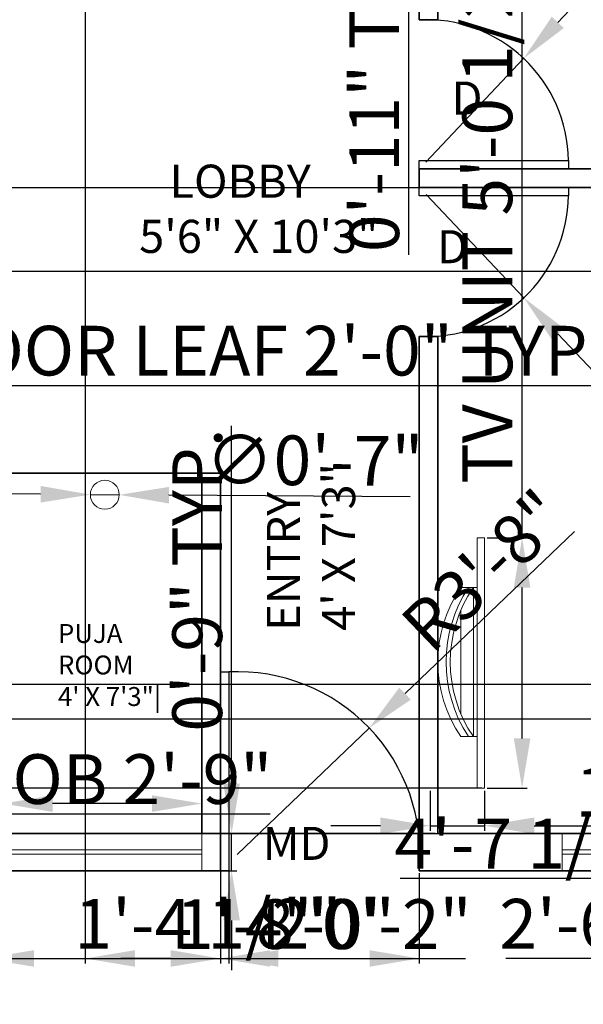
# Model space of a CAD drawing. Units: inches. Extents: x 2122 to 2726, y 1923 to 2370.
# Tile 2 of 6: x 2370 to 2506, y 1940 to 2178. Entities that reach past the tile are written whole.
import ezdxf

# ---------------------------------------------------------------- set-up
doc = ezdxf.new("R2010")
doc.units = ezdxf.units.IN
for name, color, linetype, lineweight in [('A-ANNO-DIMS', 2, 'Continuous', 18), ('A-ANNO-TEXT', 7, 'Continuous', 18), ('A-AREA-IDEN', 7, 'Continuous', 25), ('A-DOOR', 3, 'Continuous', 25), ('A-EQPM', 9, 'Continuous', 18), ('A-FLOR-FIXT', 9, 'Continuous', 18), ('A-GLAZ', 4, 'Continuous', 18), ('A-WALL', 7, 'Continuous', 35)]:
    doc.layers.add(name, color=color, linetype=linetype, lineweight=lineweight)
doc.styles.get("Standard").update_dxf_attribs({"font": 'arial.ttf'})
doc.dimstyles.new('ISO-25', dxfattribs={"dimtxt": 12, "dimasz": 12, "dimexe": 1.25, "dimexo": 0.625, "dimtad": 1, "dimlunit": 3, "dimtxsty": 'Standard', "dimcen": 2.5, "dimadec": 0, "dimazin": 0, "dimtfac": 1, "dimtmove": 0, "dimatfit": 3, "dimfxl": 1, "dimarcsym": 0})

# ---------------------------------------------------------------- blocks, each defined once
blk = doc.blocks.new('Television')
for p, q in [((2488.56, 2041.12), (2484.64, 2041.12)), ((2487.64, 2005.12), (2487.64, 2041.12)), ((2484.64, 2010.57), (2484.64, 2035.66)), ((2488.56, 2005.12), (2484.64, 2005.12))]:
    blk.add_line(p, q)
blk.add_lwpolyline([(2488.56, 2053.12), (2490.33, 2053.12), (2490.33, 1992.66), (2488.56, 1992.66)], close=True)
for centre, radius, start, end in [((2510.99, 2023.12), 31.91, 145.6614, 214.3386), ((2513.92, 2023.12), 32.85, 146.7698, 213.2302), ((2513.92, 2023.12), 31.85, 145.583, 214.417)]:
    blk.add_arc(centre, radius, start, end)
blk = doc.blocks.new('WIN-60IN')
for p, q in [((0, 0), (0, 9)), ((60, 0), (60, 9)), ((0, 5), (60, 5)), ((0, 4), (60, 4))]:
    blk.add_line(p, q)
blk = doc.blocks.new('WIN-48IN')
for p, q in [((9, 48), (0, 48)), ((4, 0), (4, 48)), ((5, 0), (5, 48)), ((9, 0), (0, 0))]:
    blk.add_line(p, q)
blk = doc.blocks.new('DOOR-LEAF-36IN')
for p, q in [((0, 2), (36, 2)), ((0, 0), (0, 2)), ((36, 0), (0, 0)), ((36, 2), (36, 0))]:
    blk.add_line(p, q)
blk = doc.blocks.new('*D18')
at = {"layer": 'A-ANNO-DIMS', "color": 0, "lineweight": -2, "transparency": 16777216}
for p, q in [((2366.01, 1982.36), (2366.01, 1990.19)), ((2414.01, 1982.36), (2414.01, 1990.19)), ((2366.01, 1988.94), (2200.91, 1988.94)), ((2402.01, 1988.94), (2378.01, 1988.94))]:
    blk.add_line(p, q, dxfattribs=at)
at = {"layer": 'A-ANNO-DIMS', "color": 0, "transparency": 16777216}
for points in [[(2378.01, 1990.94), (2378.01, 1986.94), (2366.01, 1988.94)], [(2402.01, 1990.94), (2402.01, 1986.94), (2414.01, 1988.94)]]:
    blk.add_solid(points, dxfattribs=at)
at = {"layer": 'Defpoints', "color": 0, "transparency": 16777216}
for p in [(2366.01, 1988.94), (2366.01, 1981.74), (2414.01, 1981.74)]:
    blk.add_point(p, dxfattribs=at)
at = {"layer": 'A-ANNO-DIMS', "color": 0, "transparency": 16777216, "insert": (2277.46, 1995.77), "char_height": 12, "attachment_point": 5}
blk.add_mtext('WINDOW 4\'-0" TYP.', dxfattribs=at)
blk = doc.blocks.new('*D19')
at = {"layer": 'A-ANNO-DIMS', "color": 0, "lineweight": -2, "transparency": 16777216}
for p, q in [((2421.21, 1993.74), (2421.21, 2080.13)), ((2414.63, 1981.74), (2422.46, 1981.74)), ((2421.21, 1972.74), (2421.21, 1981.74)), ((2414.63, 1972.74), (2422.46, 1972.74)), ((2421.21, 1960.74), (2421.21, 1948.74))]:
    blk.add_line(p, q, dxfattribs=at)
at = {"layer": 'A-ANNO-DIMS', "color": 0, "transparency": 16777216}
for points in [[(2419.21, 1993.74), (2423.21, 1993.74), (2421.21, 1981.74)], [(2419.21, 1960.74), (2423.21, 1960.74), (2421.21, 1972.74)]]:
    blk.add_solid(points, dxfattribs=at)
at = {"layer": 'Defpoints', "color": 0, "transparency": 16777216}
for p in [(2414.01, 1981.74), (2421.21, 1981.74), (2414.01, 1972.74)]:
    blk.add_point(p, dxfattribs=at)
at = {"layer": 'A-ANNO-DIMS', "color": 0, "transparency": 16777216, "insert": (2414.46, 2042.93), "char_height": 12, "attachment_point": 5, "rotation": 90}
blk.add_mtext('0\'-9" TYP.', dxfattribs=at)
blk = doc.blocks.new('*D24')
at = {"layer": 'A-ANNO-DIMS', "color": 0, "lineweight": -2, "transparency": 16777216}
for p, q in [((2294.01, 2092.91), (2294.01, 2088.68)), ((2318.01, 2092.91), (2318.01, 2088.68)), ((2282.01, 2089.93), (2270.01, 2089.93)), ((2294.01, 2089.93), (2318.01, 2089.93)), ((2330.01, 2089.93), (2517.34, 2089.93))]:
    blk.add_line(p, q, dxfattribs=at)
at = {"layer": 'A-ANNO-DIMS', "color": 0, "transparency": 16777216}
for points in [[(2282.01, 2091.93), (2282.01, 2087.93), (2294.01, 2089.93)], [(2330.01, 2091.93), (2330.01, 2087.93), (2318.01, 2089.93)]]:
    blk.add_solid(points, dxfattribs=at)
at = {"layer": 'Defpoints', "color": 0, "transparency": 16777216}
for p in [(2294.01, 2093.53), (2318.01, 2093.53), (2318.01, 2089.93)]:
    blk.add_point(p, dxfattribs=at)
at = {"layer": 'A-ANNO-DIMS', "color": 0, "transparency": 16777216, "insert": (2429.67, 2096.76), "char_height": 12, "attachment_point": 5}
blk.add_mtext('DOOR LEAF 2\'-0" TYP.', dxfattribs=at)
blk = doc.blocks.new('*D29')
at = {"layer": 'A-ANNO-DIMS', "color": 0, "lineweight": -2, "transparency": 16777216}
for p, q in [((2463.94, 2251.92), (2463.94, 2263.92)), ((2462.8, 2239.92), (2465.19, 2239.92)), ((2463.94, 2239.92), (2463.94, 2229.14)), ((2462.8, 2229.14), (2465.19, 2229.14)), ((2463.94, 2217.14), (2463.94, 2121.42))]:
    blk.add_line(p, q, dxfattribs=at)
at = {"layer": 'A-ANNO-DIMS', "color": 0, "transparency": 16777216}
for points in [[(2461.94, 2251.92), (2465.94, 2251.92), (2463.94, 2239.92)], [(2461.94, 2217.14), (2465.94, 2217.14), (2463.94, 2229.14)]]:
    blk.add_solid(points, dxfattribs=at)
at = {"layer": 'Defpoints', "color": 0, "transparency": 16777216}
for p in [(2462.17, 2239.92), (2462.17, 2229.14), (2463.94, 2229.14)]:
    blk.add_point(p, dxfattribs=at)
at = {"layer": 'A-ANNO-DIMS', "color": 0, "transparency": 16777216, "insert": (2457.19, 2163.28), "char_height": 12, "attachment_point": 5, "rotation": 90}
blk.add_mtext('0\'-11" TYP.', dxfattribs=at)
blk = doc.blocks.new('*D30')
at = {"layer": 'A-ANNO-DIMS', "color": 0, "lineweight": -2, "transparency": 16777216}
for p, q in [((2311.94, 1990.8), (2311.94, 1985.22)), ((2344.99, 1990.8), (2344.99, 1985.22)), ((2323.94, 1986.47), (2332.99, 1986.47)), ((2344.99, 1986.47), (2430.48, 1986.47))]:
    blk.add_line(p, q, dxfattribs=at)
at = {"layer": 'A-ANNO-DIMS', "color": 0, "transparency": 16777216}
for points in [[(2323.94, 1988.47), (2323.94, 1984.47), (2311.94, 1986.47)], [(2332.99, 1988.47), (2332.99, 1984.47), (2344.99, 1986.47)]]:
    blk.add_solid(points, dxfattribs=at)
at = {"layer": 'Defpoints', "color": 0, "transparency": 16777216}
for p in [(2311.94, 1991.43), (2344.99, 1991.43), (2344.99, 1986.47)]:
    blk.add_point(p, dxfattribs=at)
at = {"layer": 'A-ANNO-DIMS', "color": 0, "transparency": 16777216, "insert": (2393.73, 1993.3), "char_height": 12, "attachment_point": 5}
blk.add_mtext('HOB 2\'-9"', dxfattribs=at)
blk = doc.blocks.new('*D34')
at = {"layer": 'A-ANNO-DIMS', "color": 0, "lineweight": -2, "transparency": 16777216}
for p, q in [((2524.67, 2054.11), (2524.67, 2177.46)), ((2534.9, 2054.11), (2523.42, 2054.11)), ((2524.67, 1993.74), (2524.67, 2042.11)), ((2534.9, 1981.74), (2523.42, 1981.74))]:
    blk.add_line(p, q, dxfattribs=at)
at = {"layer": 'A-ANNO-DIMS', "color": 0, "transparency": 16777216}
for points in [[(2522.67, 2042.11), (2526.67, 2042.11), (2524.67, 2054.11)], [(2522.67, 1993.74), (2526.67, 1993.74), (2524.67, 1981.74)]]:
    blk.add_solid(points, dxfattribs=at)
at = {"layer": 'Defpoints', "color": 0, "transparency": 16777216}
for p in [(2524.67, 2054.11), (2535.52, 2054.11), (2535.52, 1981.74)]:
    blk.add_point(p, dxfattribs=at)
at = {"layer": 'A-ANNO-DIMS', "color": 0, "transparency": 16777216, "insert": (2517.83, 2121.79), "char_height": 12, "attachment_point": 5, "rotation": 90}
blk.add_mtext('SOFA 6\'-0 1/2"', dxfattribs=at)
blk = doc.blocks.new('*D35')
at = {"layer": 'A-ANNO-DIMS', "color": 0, "lineweight": -2, "transparency": 16777216}
for p, q in [((2535.52, 1981.11), (2535.52, 1969.63)), ((2591.01, 1981.11), (2591.01, 1969.63)), ((2535.52, 1970.88), (2461.93, 1970.88)), ((2579.01, 1970.88), (2547.52, 1970.88))]:
    blk.add_line(p, q, dxfattribs=at)
at = {"layer": 'A-ANNO-DIMS', "color": 0, "transparency": 16777216}
for points in [[(2547.52, 1972.88), (2547.52, 1968.88), (2535.52, 1970.88)], [(2579.01, 1972.88), (2579.01, 1968.88), (2591.01, 1970.88)]]:
    blk.add_solid(points, dxfattribs=at)
at = {"layer": 'Defpoints', "color": 0, "transparency": 16777216}
for p in [(2535.52, 1981.74), (2591.01, 1981.74), (2535.52, 1970.88)]:
    blk.add_point(p, dxfattribs=at)
at = {"layer": 'A-ANNO-DIMS', "color": 0, "transparency": 16777216, "insert": (2492.72, 1977.71), "char_height": 12, "attachment_point": 5}
blk.add_mtext('4\'-7 1/2"', dxfattribs=at)
blk = doc.blocks.new('*D36')
at = {"layer": 'A-ANNO-DIMS', "color": 0, "lineweight": -2, "transparency": 16777216}
for p, q in [((2491.33, 2053.12), (2491.33, 2196.38)), ((2482.88, 2053.12), (2492.58, 2053.12)), ((2491.33, 2004.66), (2491.33, 2041.12)), ((2482.88, 1992.66), (2492.58, 1992.66))]:
    blk.add_line(p, q, dxfattribs=at)
at = {"layer": 'A-ANNO-DIMS', "color": 0, "transparency": 16777216}
for points in [[(2489.33, 2041.12), (2493.33, 2041.12), (2491.33, 2053.12)], [(2489.33, 2004.66), (2493.33, 2004.66), (2491.33, 1992.66)]]:
    blk.add_solid(points, dxfattribs=at)
at = {"layer": 'Defpoints', "color": 0, "transparency": 16777216}
for p in [(2482.26, 2053.12), (2491.33, 2053.12), (2482.26, 1992.66)]:
    blk.add_point(p, dxfattribs=at)
at = {"layer": 'A-ANNO-DIMS', "color": 0, "transparency": 16777216, "insert": (2484.5, 2130.75), "char_height": 12, "attachment_point": 5, "rotation": 90}
blk.add_mtext('TV UNIT 5\'-0 1/2"', dxfattribs=at)
blk = doc.blocks.new('*D37')
at = {"layer": 'A-ANNO-DIMS', "color": 0, "lineweight": -2, "transparency": 16777216}
for p, q in [((2469.15, 1992.03), (2469.15, 1982.34)), ((2482.26, 1992.03), (2482.26, 1982.34)), ((2457.15, 1983.59), (2445.15, 1983.59)), ((2469.15, 1983.59), (2482.26, 1983.59)), ((2494.26, 1983.59), (2538.28, 1983.59))]:
    blk.add_line(p, q, dxfattribs=at)
at = {"layer": 'A-ANNO-DIMS', "color": 0, "transparency": 16777216}
for points in [[(2457.15, 1985.59), (2457.15, 1981.59), (2469.15, 1983.59)], [(2494.26, 1985.59), (2494.26, 1981.59), (2482.26, 1983.59)]]:
    blk.add_solid(points, dxfattribs=at)
at = {"layer": 'Defpoints', "color": 0, "transparency": 16777216}
for p in [(2469.15, 1992.66), (2482.26, 1992.66), (2482.26, 1983.59)]:
    blk.add_point(p, dxfattribs=at)
at = {"layer": 'A-ANNO-DIMS', "color": 0, "transparency": 16777216, "insert": (2522.27, 1990.24), "char_height": 12, "attachment_point": 5}
blk.add_mtext('1\'-1"', dxfattribs=at)
blk = doc.blocks.new('*D38')
at = {"layer": 'A-ANNO-DIMS', "color": 0, "lineweight": -2, "transparency": 16777216}
for p, q in [((2418.51, 1972.11), (2418.51, 1950.29)), ((2466.51, 1972.11), (2466.51, 1950.29)), ((2430.51, 1951.54), (2454.51, 1951.54))]:
    blk.add_line(p, q, dxfattribs=at)
at = {"layer": 'A-ANNO-DIMS', "color": 0, "transparency": 16777216}
for points in [[(2430.51, 1953.54), (2430.51, 1949.54), (2418.51, 1951.54)], [(2454.51, 1953.54), (2454.51, 1949.54), (2466.51, 1951.54)]]:
    blk.add_solid(points, dxfattribs=at)
at = {"layer": 'Defpoints', "color": 0, "transparency": 16777216}
for p in [(2418.51, 1972.74), (2466.51, 1972.74), (2466.51, 1951.54)]:
    blk.add_point(p, dxfattribs=at)
at = {"layer": 'A-ANNO-DIMS', "color": 0, "transparency": 16777216, "insert": (2442.51, 1958.29), "char_height": 12, "attachment_point": 5}
blk.add_mtext('4\'-0"', dxfattribs=at)
blk = doc.blocks.new('*D40')
at = {"layer": 'A-ANNO-DIMS', "color": 0, "lineweight": -2, "transparency": 16777216}
for p, q in [((2362.13, 2017.74), (2622.46, 2017.74)), ((2621.21, 1993.74), (2621.21, 2005.74)), ((2362.13, 1981.74), (2622.46, 1981.74))]:
    blk.add_line(p, q, dxfattribs=at)
at = {"layer": 'A-ANNO-DIMS', "color": 0, "transparency": 16777216}
for points in [[(2619.21, 2005.74), (2623.21, 2005.74), (2621.21, 2017.74)], [(2619.21, 1993.74), (2623.21, 1993.74), (2621.21, 1981.74)]]:
    blk.add_solid(points, dxfattribs=at)
at = {"layer": 'Defpoints', "color": 0, "transparency": 16777216}
for p in [(2361.51, 2017.74), (2621.21, 2017.74), (2361.51, 1981.74)]:
    blk.add_point(p, dxfattribs=at)
at = {"layer": 'A-ANNO-DIMS', "color": 0, "transparency": 16777216, "insert": (2614.45, 1999.74), "char_height": 12, "attachment_point": 5, "rotation": 90}
blk.add_mtext('3\'-0"', dxfattribs=at)
blk = doc.blocks.new('*D50')
at = {"layer": 'A-ANNO-DIMS', "color": 0, "lineweight": -2, "transparency": 16777216}
for p, q in [((2366.01, 2189.61), (2366.01, 1950.29)), ((2385.88, 2189.61), (2385.88, 1950.29)), ((2354.01, 1951.54), (2342.01, 1951.54)), ((2366.01, 1951.54), (2385.88, 1951.54)), ((2397.88, 1951.54), (2441.9, 1951.54))]:
    blk.add_line(p, q, dxfattribs=at)
at = {"layer": 'A-ANNO-DIMS', "color": 0, "transparency": 16777216}
for points in [[(2354.01, 1953.54), (2354.01, 1949.54), (2366.01, 1951.54)], [(2397.88, 1953.54), (2397.88, 1949.54), (2385.88, 1951.54)]]:
    blk.add_solid(points, dxfattribs=at)
at = {"layer": 'Defpoints', "color": 0, "transparency": 16777216}
for p in [(2366.01, 2190.24), (2385.88, 2190.24), (2385.88, 1951.54)]:
    blk.add_point(p, dxfattribs=at)
at = {"layer": 'A-ANNO-DIMS', "color": 0, "transparency": 16777216, "insert": (2425.89, 1958.29), "char_height": 12, "attachment_point": 5}
blk.add_mtext('1\'-8"', dxfattribs=at)
blk = doc.blocks.new('*D51')
at = {"layer": 'A-ANNO-DIMS', "color": 0, "lineweight": -2, "transparency": 16777216}
for p, q in [((2211.31, 2209.57), (2211.31, 2282.68)), ((2465.88, 2197.57), (2210.06, 2197.57)), ((2211.31, 2190.24), (2211.31, 2197.57)), ((2465.88, 2190.24), (2210.06, 2190.24)), ((2211.31, 2178.24), (2211.31, 2166.24))]:
    blk.add_line(p, q, dxfattribs=at)
at = {"layer": 'A-ANNO-DIMS', "color": 0, "transparency": 16777216}
for points in [[(2209.31, 2209.57), (2213.31, 2209.57), (2211.31, 2197.57)], [(2209.31, 2178.24), (2213.31, 2178.24), (2211.31, 2190.24)]]:
    blk.add_solid(points, dxfattribs=at)
at = {"layer": 'Defpoints', "color": 0, "transparency": 16777216}
for p in [(2211.31, 2197.57), (2466.51, 2197.57), (2466.51, 2190.24)]:
    blk.add_point(p, dxfattribs=at)
at = {"layer": 'A-ANNO-DIMS', "color": 0, "transparency": 16777216, "insert": (2204.48, 2252.12), "char_height": 12, "attachment_point": 5, "rotation": 90}
blk.add_mtext('0\'-7 1/2"', dxfattribs=at)
blk = doc.blocks.new('*D52')
at = {"layer": 'A-ANNO-DIMS', "color": 0, "lineweight": -2, "transparency": 16777216}
for p, q in [((2621.21, 2149.74), (2621.21, 2161.74)), ((2314.13, 2137.74), (2622.46, 2137.74)), ((2621.21, 2137.74), (2621.21, 2117.53)), ((2314.13, 2117.53), (2622.46, 2117.53)), ((2621.21, 2105.53), (2621.21, 2061.51))]:
    blk.add_line(p, q, dxfattribs=at)
at = {"layer": 'A-ANNO-DIMS', "color": 0, "transparency": 16777216}
for points in [[(2619.21, 2149.74), (2623.21, 2149.74), (2621.21, 2137.74)], [(2619.21, 2105.53), (2623.21, 2105.53), (2621.21, 2117.53)]]:
    blk.add_solid(points, dxfattribs=at)
at = {"layer": 'Defpoints', "color": 0, "transparency": 16777216}
for p in [(2313.51, 2137.74), (2313.51, 2117.53), (2621.21, 2117.53)]:
    blk.add_point(p, dxfattribs=at)
at = {"layer": 'A-ANNO-DIMS', "color": 0, "transparency": 16777216, "insert": (2614.46, 2077.52), "char_height": 12, "attachment_point": 5, "rotation": 90}
blk.add_mtext('1\'-8"', dxfattribs=at)
blk = doc.blocks.new('*D55')
at = {"layer": 'A-ANNO-DIMS', "color": 0, "lineweight": -2, "transparency": 16777216}
for p, q in [((2344.97, 1990.8), (2344.97, 1950.29)), ((2361.51, 1981.11), (2361.51, 1950.29)), ((2332.97, 1951.54), (2320.97, 1951.54)), ((2344.97, 1951.54), (2361.51, 1951.54)), ((2373.51, 1951.54), (2445.49, 1951.54))]:
    blk.add_line(p, q, dxfattribs=at)
at = {"layer": 'A-ANNO-DIMS', "color": 0, "transparency": 16777216}
for points in [[(2332.97, 1953.54), (2332.97, 1949.54), (2344.97, 1951.54)], [(2373.51, 1953.54), (2373.51, 1949.54), (2361.51, 1951.54)]]:
    blk.add_solid(points, dxfattribs=at)
at = {"layer": 'Defpoints', "color": 0, "transparency": 16777216}
for p in [(2344.97, 1991.43), (2361.51, 1981.74), (2361.51, 1951.54)]:
    blk.add_point(p, dxfattribs=at)
at = {"layer": 'A-ANNO-DIMS', "color": 0, "transparency": 16777216, "insert": (2415.5, 1958.37), "char_height": 12, "attachment_point": 5}
blk.add_mtext('1\'-4 1/2"', dxfattribs=at)
blk = doc.blocks.new('*D56')
at = {"layer": 'A-ANNO-DIMS', "color": 0, "lineweight": -2, "transparency": 16777216}
for p, q in [((2621.21, 2029.74), (2621.21, 2102.85)), ((2362.13, 2017.74), (2622.46, 2017.74)), ((2621.21, 2009.39), (2621.21, 2017.74)), ((2345.6, 2009.39), (2622.46, 2009.39)), ((2621.21, 1997.39), (2621.21, 1985.39))]:
    blk.add_line(p, q, dxfattribs=at)
at = {"layer": 'A-ANNO-DIMS', "color": 0, "transparency": 16777216}
for points in [[(2619.21, 2029.74), (2623.21, 2029.74), (2621.21, 2017.74)], [(2619.21, 1997.39), (2623.21, 1997.39), (2621.21, 2009.39)]]:
    blk.add_solid(points, dxfattribs=at)
at = {"layer": 'Defpoints', "color": 0, "transparency": 16777216}
for p in [(2361.51, 2017.74), (2621.21, 2017.74), (2344.97, 2009.39)]:
    blk.add_point(p, dxfattribs=at)
at = {"layer": 'A-ANNO-DIMS', "color": 0, "transparency": 16777216, "insert": (2614.38, 2072.29), "char_height": 12, "attachment_point": 5, "rotation": 90}
blk.add_mtext('0\'-8 1/2"', dxfattribs=at)
blk = doc.blocks.new('*D59')
at = {"layer": 'A-ANNO-DIMS', "color": 0, "lineweight": -2, "transparency": 16777216}
for p, q in [((2211.31, 2004.66), (2211.31, 2059.13)), ((2481.63, 1992.66), (2210.06, 1992.66)), ((2211.31, 1981.74), (2211.31, 1992.66)), ((2470.38, 1981.74), (2210.06, 1981.74)), ((2211.31, 1969.74), (2211.31, 1957.74))]:
    blk.add_line(p, q, dxfattribs=at)
at = {"layer": 'A-ANNO-DIMS', "color": 0, "transparency": 16777216}
for points in [[(2209.31, 2004.66), (2213.31, 2004.66), (2211.31, 1992.66)], [(2209.31, 1969.74), (2213.31, 1969.74), (2211.31, 1981.74)]]:
    blk.add_solid(points, dxfattribs=at)
at = {"layer": 'Defpoints', "color": 0, "transparency": 16777216}
for p in [(2211.31, 1992.66), (2482.26, 1992.66), (2471.01, 1981.74)]:
    blk.add_point(p, dxfattribs=at)
at = {"layer": 'A-ANNO-DIMS', "color": 0, "transparency": 16777216, "insert": (2204.56, 2037.89), "char_height": 12, "attachment_point": 5, "rotation": 90}
blk.add_mtext('0\'-11"', dxfattribs=at)
blk = doc.blocks.new('*D62')
at = {"layer": 'A-ANNO-DIMS', "color": 0, "lineweight": -2, "transparency": 16777216}
for p, q in [((2560.71, 2148.71), (2560.71, 1950.29)), ((2591.01, 2141.61), (2591.01, 1950.29)), ((2560.71, 1951.54), (2487.39, 1951.54)), ((2579.01, 1951.54), (2572.71, 1951.54))]:
    blk.add_line(p, q, dxfattribs=at)
at = {"layer": 'A-ANNO-DIMS', "color": 0, "transparency": 16777216}
for points in [[(2572.71, 1953.54), (2572.71, 1949.54), (2560.71, 1951.54)], [(2579.01, 1953.54), (2579.01, 1949.54), (2591.01, 1951.54)]]:
    blk.add_solid(points, dxfattribs=at)
at = {"layer": 'Defpoints', "color": 0, "transparency": 16777216}
for p in [(2560.71, 2149.34), (2591.01, 2142.24), (2560.71, 1951.54)]:
    blk.add_point(p, dxfattribs=at)
at = {"layer": 'A-ANNO-DIMS', "color": 0, "transparency": 16777216, "insert": (2518.05, 1958.37), "char_height": 12, "attachment_point": 5}
blk.add_mtext('2\'-6 1/2"', dxfattribs=at)
blk = doc.blocks.new('*D65')
at = {"layer": 'A-ANNO-DIMS', "color": 0, "lineweight": -2, "transparency": 16777216}
for p, q in [((2211.31, 2274.24), (2211.31, 2286.24)), ((2413.38, 2262.24), (2210.06, 2262.24)), ((2211.31, 2262.24), (2211.31, 2238.81)), ((2409.54, 2238.81), (2210.06, 2238.81)), ((2211.31, 2226.81), (2211.31, 2145.5))]:
    blk.add_line(p, q, dxfattribs=at)
at = {"layer": 'A-ANNO-DIMS', "color": 0, "transparency": 16777216}
for points in [[(2209.31, 2274.24), (2213.31, 2274.24), (2211.31, 2262.24)], [(2209.31, 2226.81), (2213.31, 2226.81), (2211.31, 2238.81)]]:
    blk.add_solid(points, dxfattribs=at)
at = {"layer": 'Defpoints', "color": 0, "transparency": 16777216}
for p in [(2414.01, 2262.24), (2211.31, 2238.81), (2410.17, 2238.81)]:
    blk.add_point(p, dxfattribs=at)
at = {"layer": 'A-ANNO-DIMS', "color": 0, "transparency": 16777216, "insert": (2204.48, 2180.16), "char_height": 12, "attachment_point": 5, "rotation": 90}
blk.add_mtext('1\'-11 1/2"', dxfattribs=at)
blk = doc.blocks.new('*D68')
at = {"layer": 'A-ANNO-DIMS', "color": 0, "lineweight": -2, "transparency": 16777216}
for p, q in [((2418.51, 2020.11), (2418.51, 1950.29)), ((2420.51, 2020.11), (2420.51, 1950.29)), ((2406.51, 1951.54), (2394.51, 1951.54)), ((2418.51, 1951.54), (2420.51, 1951.54)), ((2432.51, 1951.54), (2477.66, 1951.54))]:
    blk.add_line(p, q, dxfattribs=at)
at = {"layer": 'A-ANNO-DIMS', "color": 0, "transparency": 16777216}
for points in [[(2406.51, 1953.54), (2406.51, 1949.54), (2418.51, 1951.54)], [(2432.51, 1953.54), (2432.51, 1949.54), (2420.51, 1951.54)]]:
    blk.add_solid(points, dxfattribs=at)
at = {"layer": 'Defpoints', "color": 0, "transparency": 16777216}
for p in [(2418.51, 2020.74), (2420.51, 2020.74), (2420.51, 1951.54)]:
    blk.add_point(p, dxfattribs=at)
at = {"layer": 'A-ANNO-DIMS', "color": 0, "transparency": 16777216, "insert": (2461.08, 1958.29), "char_height": 12, "attachment_point": 5}
blk.add_mtext('0\'-2"', dxfattribs=at)
blk = doc.blocks.new('*D69')
at = {"layer": 'A-ANNO-DIMS', "color": 0, "lineweight": -2, "transparency": 16777216}
for p, q in [((2503.97, 2054.68), (2463.08, 2015.5)), ((2422.57, 1976.67), (2454.42, 2007.19))]:
    blk.add_line(p, q, dxfattribs=at)
at = {"layer": 'A-ANNO-DIMS', "color": 0, "transparency": 16777216}
blk.add_solid([(2461.7, 2016.94), (2464.47, 2014.05), (2454.42, 2007.19)], dxfattribs=at)
at = {"layer": 'Defpoints', "color": 0, "transparency": 16777216}
for p in [(2454.42, 2007.19), (2422.57, 1976.67)]:
    blk.add_point(p, dxfattribs=at)
at = {"layer": 'A-ANNO-DIMS', "color": 0, "transparency": 16777216, "insert": (2483.19, 2044.12), "char_height": 12, "attachment_point": 5, "rotation": 43.7813}
blk.add_mtext('R3\'-8"', dxfattribs=at)
blk = doc.blocks.new('*D71')
at = {"layer": 'A-ANNO-DIMS', "color": 0, "lineweight": -2, "transparency": 16777216}
for p, q in [((2564.44, 2245.87), (2499.95, 2177.59)), ((2468.06, 2143.82), (2491.71, 2168.87))]:
    blk.add_line(p, q, dxfattribs=at)
at = {"layer": 'A-ANNO-DIMS', "color": 0, "transparency": 16777216}
blk.add_solid([(2498.5, 2178.96), (2501.41, 2176.22), (2491.71, 2168.87)], dxfattribs=at)
at = {"layer": 'Defpoints', "color": 0, "transparency": 16777216}
for p in [(2491.71, 2168.87), (2468.06, 2143.82)]:
    blk.add_point(p, dxfattribs=at)
at = {"layer": 'A-ANNO-DIMS', "color": 0, "transparency": 16777216, "insert": (2531.35, 2220.78), "char_height": 12, "attachment_point": 5, "rotation": 46.6362}
blk.add_mtext('R2\'-10 1/2"', dxfattribs=at)
blk = doc.blocks.new('*D72')
at = {"layer": 'A-ANNO-DIMS', "color": 0, "lineweight": -2, "transparency": 16777216}
for p, q in [((2468.16, 2136.04), (2491.75, 2111.07)), ((2564.47, 2034.07), (2499.99, 2102.35))]:
    blk.add_line(p, q, dxfattribs=at)
at = {"layer": 'A-ANNO-DIMS', "color": 0, "transparency": 16777216}
blk.add_solid([(2501.44, 2103.72), (2498.53, 2100.97), (2491.75, 2111.07)], dxfattribs=at)
at = {"layer": 'Defpoints', "color": 0, "transparency": 16777216}
for p in [(2468.16, 2136.04), (2491.75, 2111.07)]:
    blk.add_point(p, dxfattribs=at)
at = {"layer": 'A-ANNO-DIMS', "color": 0, "transparency": 16777216, "insert": (2541.31, 2068.53), "char_height": 12, "attachment_point": 5, "rotation": 313.3635}
blk.add_mtext('R2\'-10 1/2"', dxfattribs=at)
blk = doc.blocks.new('*D76')
at = {"layer": 'A-ANNO-DIMS', "color": 0, "lineweight": -2, "transparency": 16777216}
for p, q in [((2375.12, 2063.64), (2363.12, 2063.73)), ((2387.12, 2063.55), (2394.08, 2063.5)), ((2464.28, 2062.99), (2406.08, 2063.41))]:
    blk.add_line(p, q, dxfattribs=at)
at = {"layer": 'A-ANNO-DIMS', "color": 0, "transparency": 16777216}
for points in [[(2375.13, 2065.64), (2375.1, 2061.64), (2387.12, 2063.55)], [(2406.09, 2065.41), (2406.07, 2061.41), (2394.08, 2063.5)]]:
    blk.add_solid(points, dxfattribs=at)
at = {"layer": 'Defpoints', "color": 0, "transparency": 16777216}
for p in [(2387.12, 2063.55), (2394.08, 2063.5)]:
    blk.add_point(p, dxfattribs=at)
at = {"layer": 'A-ANNO-DIMS', "color": 0, "transparency": 16777216, "insert": (2441.23, 2070.24), "char_height": 12, "attachment_point": 5, "rotation": 359.5814}
blk.add_mtext('∅0\'-7"', dxfattribs=at)

msp = doc.modelspace()

# ---------------------------------------------------------------- linework, layer by layer
at = {"layer": 'A-DOOR'}
for p, q in [((2418.508, 1972.736), (2418.508, 2020.736)), ((2418.508, 2020.736), (2420.508, 2020.736)), ((2420.508, 2020.736), (2420.508, 1972.736)), ((2420.508, 1972.736), (2418.508, 1972.736))]:
    msp.add_line(p, q, dxfattribs=at)
for centre, radius, start, end in [((2468.058, 2143.819), 34.452, 0.69324, 92.57991), ((2468.165, 2136.04), 34.344, 267.23449, 359.49236), ((2422.572, 1976.673), 44.112, 354.87999, 92.68226)]:
    msp.add_arc(centre, radius, start, end, dxfattribs=at)
at = {"layer": 'A-FLOR-FIXT'}
msp.add_circle((2390.6, 2063.525), 3.481, dxfattribs=at)
at = {"layer": 'A-WALL'}
for p, q in [((2471.008, 2178.236), (2471.008, 2197.569)), ((2466.508, 2178.236), (2466.508, 2185.736)), ((2471.008, 2178.236), (2466.508, 2178.236)), ((2466.508, 2137.736), (2466.508, 2142.236)), ((2471.008, 2142.236), (2466.508, 2142.236)), ((2471.008, 2142.236), (2591.008, 2142.236)), ((2471.008, 2137.736), (2466.508, 2137.736)), ((2471.008, 2137.736), (2591.008, 2137.736)), ((2466.508, 1981.736), (2466.508, 2101.736)), ((2471.008, 2101.736), (2466.508, 2101.736)), ((2471.008, 2101.736), (2471.008, 1981.736)), ((2418.508, 2068.736), (2361.508, 2068.736)), ((2414.008, 2068.736), (2414.008, 1981.736)), ((2418.508, 2068.736), (2418.508, 1981.736)), ((2414.008, 1981.736), (2366.008, 1981.736)), ((2418.508, 1981.736), (2418.508, 1972.736)), ((2466.508, 1981.736), (2466.508, 1972.736)), ((2471.008, 1981.736), (2591.008, 1981.736)), ((2418.508, 1972.736), (2232.508, 1972.736)), ((2471.008, 1972.736), (2466.508, 1972.736)), ((2471.008, 1972.736), (2600.008, 1972.736))]:
    msp.add_line(p, q, dxfattribs=at)

# ---------------------------------------------------------------- block references
at = {"layer": 'A-DOOR', "rotation": 180}
msp.add_blockref('DOOR-LEAF-36IN', (2502.507, 2144.236), dxfattribs=at)
at = {"layer": 'A-DOOR'}
msp.add_blockref('DOOR-LEAF-36IN', (2466.508, 2135.736), dxfattribs=at)
at = {"layer": 'A-EQPM'}
msp.add_blockref('Television', (-8.076, 0), dxfattribs=at)
at = {"layer": 'A-GLAZ', "rotation": 89.99999999999747}
msp.add_blockref('WIN-48IN', (2414.008, 1972.736), dxfattribs=at)
at = {"layer": 'A-GLAZ'}
msp.add_blockref('WIN-60IN', (2501.008, 1972.736), dxfattribs=at)

# ---------------------------------------------------------------- texts
at = {"layer": 'A-ANNO-TEXT', "attachment_point": 1}
for s, insert, char_height in [('D', (2474.286, 2163.3), 7.99), ('D', (2470.783, 2127.408), 7.99), ('MD', (2428.727, 1983.327), 7.9897)]:
    msp.add_mtext_dynamic_manual_height_columns(s, width=65.06795, gutter_width=39.949, heights=[0], dxfattribs=dict(at, insert=insert, char_height=char_height))
at = {"layer": 'A-AREA-IDEN', "attachment_point": 1}
for s, width, gutter_width, insert, char_height in [('   LOBBY \\P5\'6" X 10\'3"', 65.06795, 39.949, (2398.897, 2143.225), 7.98971), ('PUJA \\PROOM\\P4\' X 7\'3"|', 37.18666, 22.831, (2379.3, 2032.304), 4.5662)]:
    msp.add_mtext_dynamic_manual_height_columns(s, width=width, gutter_width=gutter_width, heights=[0], dxfattribs=dict(at, insert=insert, char_height=char_height))
at = {"layer": 'A-AREA-IDEN', "insert": (2429.722, 2030.679), "char_height": 7.9897, "attachment_point": 1, "rotation": 90}
msp.add_mtext_dynamic_manual_height_columns('ENTRY \\P4\' X 7\'3"', width=65.06795, gutter_width=39.949, heights=[0], dxfattribs=at)

# ---------------------------------------------------------------- dimensions: what is measured, and where the dimension line sits
at = {"layer": 'A-ANNO-DIMS'}
for base, p1, p2, angle, picture, middle in [((2211.308, 2238.809), (2414.008, 2262.236), (2410.167, 2238.809), 90, '*D65', (2204.478, 2180.156)), ((2211.308, 2197.569), (2466.508, 2190.236), (2466.508, 2197.569), 90, '*D51', (2204.478, 2252.124)), ((2621.208, 2117.531), (2313.508, 2137.736), (2313.508, 2117.531), 90, '*D52', (2614.456, 2077.521)), ((2621.208, 2017.736), (2344.971, 2009.385), (2361.508, 2017.736), 90, '*D56', (2614.378, 2072.291)), ((2211.308, 1992.656), (2471.008, 1981.736), (2482.256, 1992.656), 90, '*D59', (2204.556, 2037.893)), ((2621.208, 2017.736), (2361.508, 1981.736), (2361.508, 2017.736), 90, '*D40', (2614.452, 1999.736)), ((2535.521, 1970.88), (2591.008, 1981.736), (2535.521, 1981.736), 180, '*D35', (2492.724, 1977.71))]:
    dim = msp.add_linear_dim(base=base, p1=p1, p2=p2, angle=angle, dimstyle='ISO-25', override={"dimdec": 1, "dimlfac": 1, "dimrnd": 0, "dimzin": 1, "dimdsep": 46, "dimlunit": 4, "dimfrac": 2}, dxfattribs=at)
    dim.commit()
    dim.dimension.update_dxf_attribs({"geometry": picture, "text_midpoint": middle})
for base, p1, p2, angle, text, picture, middle in [((2463.938, 2229.14), (2462.172, 2239.919), (2462.172, 2229.14), 270, '<> TYP.', '*D29', (2457.186, 2163.28)), ((2491.325, 2053.118), (2482.256, 1992.656), (2482.256, 2053.118), 90, 'TV UNIT <>', '*D36', (2484.496, 2130.749)), ((2524.665, 2054.11), (2535.521, 1981.736), (2535.521, 2054.11), 90, 'SOFA <>', '*D34', (2517.831, 2121.787)), ((2421.208, 1981.736), (2414.008, 1972.736), (2414.008, 1981.736), 90, '<> TYP.', '*D19', (2414.456, 2042.934)), ((2366.008, 1988.936), (2414.008, 1981.736), (2366.008, 1981.736), 180, 'WINDOW <> TYP.', '*D18', (2277.458, 1995.77))]:
    dim = msp.add_linear_dim(base=base, p1=p1, p2=p2, angle=angle, text=text, dimstyle='ISO-25', override={"dimdec": 1, "dimlfac": 1, "dimrnd": 0, "dimzin": 1, "dimdsep": 46, "dimlunit": 4, "dimfrac": 2}, dxfattribs=at)
    dim.commit()
    dim.dimension.update_dxf_attribs({"geometry": picture, "text_midpoint": middle})
for center, mpoint, picture, middle in [((2468.058, 2143.819), (2491.714, 2168.866), '*D71', (2531.352, 2220.781)), ((2468.165, 2136.04), (2491.746, 2111.072), '*D72', (2541.314, 2068.535)), ((2422.572, 1976.673), (2454.42, 2007.194), '*D69', (2483.185, 2044.119))]:
    dim = msp.add_radius_dim(center=center, mpoint=mpoint, dimstyle='ISO-25', override={"dimdec": 1, "dimlfac": 1, "dimrnd": 0, "dimzin": 1, "dimdsep": 46, "dimlunit": 4, "dimfrac": 2}, dxfattribs=at)
    dim.commit()
    dim.dimension.update_dxf_attribs({"geometry": picture, "text_midpoint": middle})
for base, p1, p2, picture, middle in [((2385.877, 1951.536), (2366.008, 2190.236), (2385.877, 2190.236), '*D50', (2425.886, 1958.288)), ((2560.71, 1951.536), (2591.008, 2142.236), (2560.71, 2149.338), '*D62', (2518.053, 1958.366)), ((2420.508, 1951.536), (2418.508, 2020.736), (2420.508, 2020.736), '*D68', (2461.082, 1958.288)), ((2482.256, 1983.587), (2469.154, 1992.656), (2482.256, 1992.656), '*D37', (2522.266, 1990.237)), ((2361.508, 1951.536), (2344.971, 1991.428), (2361.508, 1981.736), '*D55', (2415.498, 1958.366)), ((2466.508, 1951.536), (2418.508, 1972.736), (2466.508, 1972.736), '*D38', (2442.508, 1958.288))]:
    dim = msp.add_linear_dim(base=base, p1=p1, p2=p2, dimstyle='ISO-25', override={"dimdec": 1, "dimlfac": 1, "dimrnd": 0, "dimzin": 1, "dimdsep": 46, "dimlunit": 4, "dimfrac": 2}, dxfattribs=at)
    dim.commit()
    dim.dimension.update_dxf_attribs({"geometry": picture, "text_midpoint": middle})
for base, p1, p2, text, picture, middle in [((2318.008, 2089.931), (2294.008, 2093.531), (2318.008, 2093.531), 'DOOR LEAF <> TYP.', '*D24', (2429.674, 2096.764)), ((2344.991, 1986.471), (2311.944, 1991.428), (2344.991, 1991.428), 'HOB <>', '*D30', (2393.735, 1993.304))]:
    dim = msp.add_linear_dim(base=base, p1=p1, p2=p2, text=text, dimstyle='ISO-25', override={"dimdec": 1, "dimlfac": 1, "dimrnd": 0, "dimzin": 1, "dimdsep": 46, "dimlunit": 4, "dimfrac": 2}, dxfattribs=at)
    dim.commit()
    dim.dimension.update_dxf_attribs({"geometry": picture, "text_midpoint": middle})
dim = msp.add_diameter_dim_2p(p1=(2387.119, 2063.55), p2=(2394.08, 2063.499), dimstyle='ISO-25', override={"dimdec": 1, "dimlfac": 1, "dimrnd": 0, "dimzin": 1, "dimdsep": 46, "dimlunit": 4, "dimfrac": 2}, dxfattribs=at)
dim.commit()
dim.dimension.update_dxf_attribs({"geometry": '*D76', "text_midpoint": (2441.182, 2063.155)})

doc.saveas('drawing.dxf')
